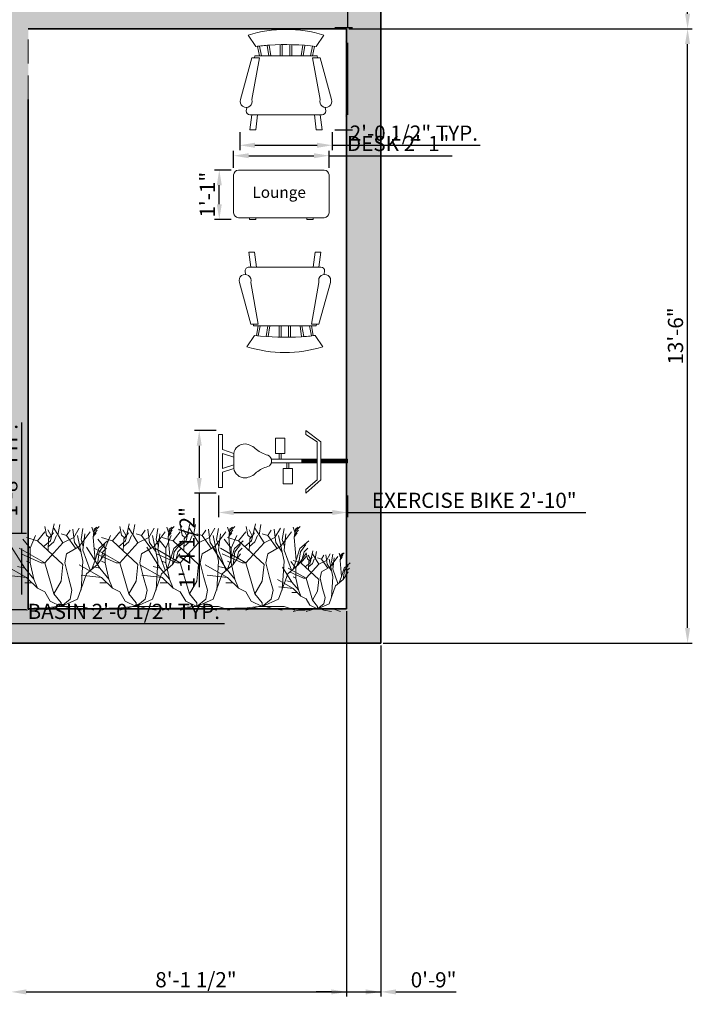
# Model space of a CAD drawing. Units: inches. Extents: x 1872 to 2380, y 714 to 1327.
# Tile 3 of 9: x 2200 to 2378, y 714 to 974. Entities that reach past the tile are written whole.
import ezdxf

# ---------------------------------------------------------------- set-up
doc = ezdxf.new("R2010")
doc.units = ezdxf.units.IN
doc.linetypes.add('HIDDEN', pattern=[9.525, 6.35, -3.175])
for name, color, linetype, lineweight in [('A-ANNO-DIMS', 2, 'Continuous', 18), ('A-AREA-IDEN', 7, 'Continuous', 18), ('A-EQPM', 8, 'Continuous', 18), ('A-FURN', 8, 'Continuous', 18), ('A-WALL', 7, 'Continuous', 35), ('A-WALL-HIDN', 7, 'HIDDEN', 18), ('L-PLNT', 3, 'Continuous', 13)]:
    doc.layers.add(name, color=color, linetype=linetype, lineweight=lineweight)
doc.layers.add('A-WALL-PATT', color=242, linetype='Continuous', lineweight=13, true_color=0xd52e31)
doc.styles.get("Standard").update_dxf_attribs({"font": 'arial.ttf'})
doc.dimstyles.new('ISO-25', dxfattribs={"dimtxt": 4, "dimasz": 4, "dimexe": 1.25, "dimexo": 0.625, "dimtad": 1, "dimdec": 0, "dimlunit": 3, "dimtxsty": 'Standard', "dimcen": 2.5, "dimadec": 0, "dimazin": 0, "dimtfac": 1, "dimtdec": 0, "dimtmove": 0, "dimatfit": 3, "dimfxl": 1, "dimarcsym": 0})

# ---------------------------------------------------------------- blocks, each defined once
blk = doc.blocks.new('*U18')
for p, q in [((-316.7634, 502.285), (-327.6092, 559.9176)), ((-286.512, 498.3226), (-307.4416, 538.0736)), ((-290.3982, 464.5406), (-265.6078, 577.8246)), ((-207.264, 451.104), (-268.224, 548.64)), ((-240.792, 502.285), (-228.3968, 573.8368)), ((-182.88, 499.872), (-158.496, 536.448)), ((-129.1844, 450.6214), (-140.0302, 542.036)), ((-134.112, 487.68), (-97.536, 548.64)), ((-85.7758, 472.4908), (-73.3552, 548.005)), ((-12.9032, 555.9552), (-2.0574, 522.1732)), ((-5.1562, 486.3846), (2.5908, 542.036)), ((-0.508, 508.254), (22.7584, 536.067)), ((1.0414, 526.1356), (35.1536, 559.9176)), ((2.5908, 542.036), (21.209, 555.9552)), ((-426.72, 414.528), (-475.488, 475.488)), ((-377.952, 463.296), (-451.104, 487.68)), ((-426.72, 414.528), (-390.144, 499.872)), ((-377.952, 463.296), (-329.184, 524.256)), ((-207.264, 304.8), (-377.952, 463.296)), ((-338.455, 424.7896), (-290.3982, 464.5406)), ((-296.5958, 484.4034), (-316.7634, 502.285)), ((-305.8922, 396.9512), (-302.7934, 478.4344)), ((-302.7934, 478.4344), (-270.256, 518.1854)), ((-268.7066, 458.5716), (-250.0884, 500.3038)), ((-182.88, 499.872), (-219.456, 512.064)), ((-207.264, 451.104), (-134.112, 487.68)), ((-121.92, 414.528), (-182.88, 499.872)), ((-73.152, 329.184), (-109.728, 499.872)), ((-97.536, 426.72), (-24.384, 524.256)), ((-70.2564, 426.7708), (-85.7758, 472.4908)), ((-73.152, 402.336), (-60.96, 512.064)), ((8.7884, 335.3562), (-5.1562, 486.3846)), ((-3.6068, 492.3536), (14.986, 518.1854)), ((33.6042, 412.8516), (92.5068, 464.5406)), ((-463.296, 280.416), (-552.577, 423.037)), ((-329.184, 316.992), (-499.872, 414.528)), ((-426.72, 316.992), (-426.72, 414.528)), ((-329.184, 316.992), (-207.264, 451.104)), ((-304.3428, 426.7708), (-268.7066, 458.5716)), ((-182.88, 377.952), (-97.536, 426.72)), ((-85.7758, 389.001), (-129.1844, 452.6026)), ((-24.384, 268.224), (-73.152, 402.336)), ((8.7884, 335.3562), (33.6042, 412.8516)), ((36.576, 390.144), (73.152, 438.912)), ((60.96, 390.144), (85.344, 414.528)), ((-353.568, 316.992), (-487.68, 377.952)), ((-195.072, 316.992), (-182.88, 377.952)), ((-12.192, 274.32), (8.7884, 335.3562)), ((24.384, 304.8), (36.576, 390.144)), ((24.384, 304.8), (73.152, 377.952)), ((48.768, 341.376), (60.96, 390.144)), ((-451.104, 219.456), (-601.0402, 303.8094)), ((-463.296, 280.416), (-512.064, 292.608)), ((-402.336, 207.264), (-463.296, 280.416)), ((-426.72, 316.992), (-451.104, 329.184)), ((-402.336, 207.264), (-426.72, 316.992)), ((-329.184, 316.992), (-353.568, 316.992)), ((-268.224, 109.728), (-329.184, 316.992)), ((-219.456, 195.072), (-207.264, 304.8)), ((-170.688, 219.456), (-195.072, 316.992)), ((-85.344, 134.112), (-73.152, 329.184)), ((-48.768, 243.84), (24.384, 304.8)), ((-451.104, 219.456), (-587.4512, 234.2388)), ((-377.952, 146.304), (-451.104, 219.456)), ((-377.952, 146.304), (-402.336, 207.264)), ((-146.304, 134.112), (-170.688, 219.456)), ((-109.728, 73.152), (-48.768, 243.84)), ((-414.528, 182.88), (-463.296, 182.88)), ((-329.184, 121.92), (-377.952, 146.304)), ((-268.224, 109.728), (-219.456, 195.072)), ((-158.496, 73.152), (-146.304, 134.112)), ((-292.608, 60.96), (-329.184, 121.92)), ((-219.456, 48.768), (-268.224, 109.728)), ((-219.456, 24.384), (-109.728, 73.152)), ((-219.456, 24.384), (-158.496, 73.152)), ((-402.336, 12.192), (-451.104, 0)), ((-341.376, 12.192), (-402.336, 12.192)), ((-243.84, 24.384), (-341.376, 12.192)), ((-243.84, 24.384), (-329.184, 0)), ((-219.456, 24.384), (-292.608, 60.96)), ((-243.84, 24.384), (-195.072, 24.384)), ((-219.456, 24.384), (-219.456, 48.768)), ((-219.456, 24.384), (-73.152, 24.384)), ((-195.072, 24.384), (-158.496, 12.192)), ((-158.496, 12.192), (-85.344, 0)), ((-73.152, 24.384), (0, 0))]:
    blk.add_line(p, q)
blk = doc.blocks.new('Desk - 30 x 60 in.')
for p, q in [((-26.999995, 0), (26.999995, 0)), ((-29.999995, -27), (-29.999995, -3)), ((29.999995, -3), (29.999995, -27)), ((26.999995, -30), (-26.999995, -30)), ((-20.000005, -30), (-20.000005, -31)), ((-16.000005, -31), (-16.000005, -30)), ((15.999995, -31), (15.999995, -30)), ((19.999995, -30), (19.999995, -31)), ((-20.000005, -31), (-16.000005, -31)), ((19.999995, -31), (15.999995, -31))]:
    blk.add_line(p, q)
for centre, start, end in [((-26.499995, -3.5), 98.1301, 171.8699), ((26.499995, -3.5), 8.130102, 81.8699), ((-26.499995, -26.5), 188.1301, 261.8699), ((26.499995, -26.5), 278.1301, 351.8699)]:
    blk.add_arc(centre, 3.535534, start, end)
blk = doc.blocks.new('Exercise Bike')
for p, q in [((-0.75, 10), (-0.75, 17)), ((-0.75, 17), (0.25, 17)), ((-0.5, 17), (-0.5, 9.9929)), ((-0.25, 10), (-0.25, 17)), ((0, 17), (0, 9.9929)), ((0.25, 17), (0.25, 10)), ((-5.25, 10), (-8.25, 6)), ((-7.25, 6), (-5.25, 9)), ((-0.75, 10), (-5.25, 10)), ((-5.25, 9), (4.75, 9)), ((4.75, 10), (-0.75, 10)), ((-0.75, 5), (-0.75, 9)), ((-0.5, 8.9396), (-0.5, 5)), ((-0.25, 5), (-0.25, 9)), ((0, 8.9396), (0, 5)), ((0.25, 9), (0.25, 5)), ((8.25, 6), (4.75, 10)), ((4.75, 9), (7.25, 6)), ((-8.25, 6), (-7.25, 6)), ((7.25, 6), (8.25, 6)), ((-0.75, -3.0635), (-0.75, 5)), ((-0.75, 5), (0.25, 5)), ((0.25, 5), (0.25, -3.0635)), ((-6.25, -2), (-6.25, 0.5)), ((-2.25, 0.5), (-6.25, 0.5)), ((-2.25, -0.5), (-2.25, 0.5)), ((0.25, 1.5), (1.75, 1.5)), ((0.25, 1), (1.75, 1)), ((1.75, 2.5), (5.75, 2.5)), ((1.75, 1.5), (1.75, 2.5)), ((1.75, 1.5), (1.75, 0)), ((1.75, 0), (5.75, 0)), ((5.75, 2.5), (5.75, 0)), ((-2.25, -2), (-6.25, -2)), ((-2.25, -0.5), (-0.75, -0.5)), ((-2.25, -1), (-2.25, -0.5)), ((-2.25, -1), (-2.25, -2)), ((-0.75, -1), (-2.25, -1)), ((-2.25, -13), (-3.25, -16)), ((-2.25, -16), (-1.25, -13)), ((-2.25, -13), (1.75, -13)), ((0.75, -13), (1.75, -16)), ((1.75, -13), (2.75, -16)), ((-7.25, -16), (-7.25, -17)), ((-4.75, -16), (-7.25, -16)), ((-7.25, -17), (6.75, -17)), ((-3.25, -16), (-4.75, -16)), ((1.75, -16), (-2.25, -16)), ((6.75, -16), (2.75, -16)), ((6.75, -17), (6.75, -16))]:
    blk.add_line(p, q)
for centre, radius, start, end in [((-9.6692, -1.9154), 8.1889, 321.6175, 345.2525), ((-0.25, -4.625), 1.625, 22.61987, 157.3801), ((9.1691, -1.9154), 8.1889, 194.7476, 218.3825), ((0.1685, -10.5843), 4.9531, 133.6443, 173.2256), ((-0.6686, -10.5843), 4.9531, 6.774486, 46.35562), ((-1.7006, -10.0005), 3.0494, 179.9906, 259.6205), ((1.2006, -10.0005), 3.0494, 280.3795, 0.009389)]:
    blk.add_arc(centre, radius, start, end)
blk = doc.blocks.new('Chair - Rocking')
for p, q in [((-8, -4.5), (-10, -1.5)), ((8, -4.5), (10, -1.5)), ((-7.5, -4.5), (-7, -7)), ((-6.5, -7), (-7.02225, -4.43)), ((-4.5, -7), (-4.96674, -4.19951)), ((-4, -7), (-4.40532, -4.16272)), ((-1.5, -4.05012), (-1.5, -7)), ((-1, -7), (-1, -4.05012)), ((1, -7), (1, -4.04655)), ((1.5, -4.05012), (1.5, -7)), ((4, -7), (4.40187, -4.18694)), ((4.5, -7), (4.96761, -4.19437)), ((6.5, -7), (7, -4.4057)), ((7.5, -4.5), (7, -7)), ((-9, -7.5), (-12, -18.49999)), ((-7, -7.5), (-9, -7.5)), ((-9, -18.49999), (-7, -7.5)), ((-8.23428, -6.99939), (-8.3093, -7.47958)), ((-8.23041, -7), (8.23915, -7)), ((7, -7.5), (9, -7.5)), ((9, -18.49999), (7, -7.5)), ((8.31071, -7.48854), (8.23449, -7.00073)), ((9, -7.5), (12, -18.49999)), ((-10.36644, -20.64523), (-10.5, -21.49999)), ((10.5, -21.49999), (10.3575, -20.58798)), ((-9, -22.49999), (-9.5, -26.49999)), ((0, -22.49999), (-9.5, -22.49999)), ((-8, -26.49999), (-7.5, -22.49999)), ((0, -22.49999), (9.5, -22.49999)), ((8, -26.49999), (7.5, -22.49999)), ((9, -22.49999), (9.5, -26.49999)), ((-9.5, -26.49999), (-8, -26.49999)), ((9.5, -26.49999), (8, -26.49999))]:
    blk.add_line(p, q)
for centre, radius, start, end in [((0, -34.08333), 34.08333, 72.93847, 107.0615), ((0, -68.25004), 64.25, 93.92211, 97.15267), ((0, -68.25004), 64.25, 82.84733, 93.92211), ((-10.5, -18.99999), 1.58114, 161.5651, 18.43495), ((10.5, -18.99999), 1.58114, 161.5651, 18.43495), ((-9.5, -21.49999), 1, 180, 270), ((9.5, -21.49999), 1, 270, 0)]:
    blk.add_arc(centre, radius, start, end)
blk = doc.blocks.new('*D30')
at = {"layer": 'A-ANNO-DIMS', "color": 0, "lineweight": -2, "transparency": 16777216}
for p, q in [((2172.51, 817.84), (2172.51, 813.54)), ((2197.06, 817.84), (2197.06, 813.54)), ((2176.51, 814.79), (2193.06, 814.79)), ((2197.06, 814.79), (2254.16, 814.79))]:
    blk.add_line(p, q, dxfattribs=at)
at = {"layer": 'A-ANNO-DIMS', "color": 0, "transparency": 16777216}
for points in [[(2176.51, 815.45), (2176.51, 814.12), (2172.51, 814.79)], [(2193.06, 815.45), (2193.06, 814.12), (2197.06, 814.79)]]:
    blk.add_solid(points, dxfattribs=at)
at = {"layer": 'Defpoints', "color": 0, "transparency": 16777216}
for p in [(2172.51, 818.47), (2197.06, 818.47), (2197.06, 814.79)]:
    blk.add_point(p, dxfattribs=at)
at = {"layer": 'A-ANNO-DIMS', "color": 0, "transparency": 16777216, "insert": (2227.61, 817.48), "char_height": 4, "attachment_point": 5}
blk.add_mtext('BASIN 2\'-0 1/2" TYP.', dxfattribs=at)
blk = doc.blocks.new('*D31')
at = {"layer": 'A-ANNO-DIMS', "color": 0, "lineweight": -2, "transparency": 16777216}
for p, q in [((2200.74, 838.61), (2200.74, 867.86)), ((2197.68, 838.61), (2201.99, 838.61)), ((2200.74, 822.47), (2200.74, 834.61)), ((2197.68, 818.47), (2201.99, 818.47))]:
    blk.add_line(p, q, dxfattribs=at)
at = {"layer": 'A-ANNO-DIMS', "color": 0, "transparency": 16777216}
for points in [[(2200.07, 834.61), (2201.41, 834.61), (2200.74, 838.61)], [(2200.07, 822.47), (2201.41, 822.47), (2200.74, 818.47)]]:
    blk.add_solid(points, dxfattribs=at)
at = {"layer": 'Defpoints', "color": 0, "transparency": 16777216}
for p in [(2197.06, 838.61), (2200.74, 838.61), (2197.06, 818.47)]:
    blk.add_point(p, dxfattribs=at)
at = {"layer": 'A-ANNO-DIMS', "color": 0, "transparency": 16777216, "insert": (2198.07, 855.23), "char_height": 4, "attachment_point": 5, "rotation": 90}
blk.add_mtext('1\'-8" TYP.', dxfattribs=at)
blk = doc.blocks.new('*D38')
at = {"layer": 'A-ANNO-DIMS', "color": 0, "lineweight": -2, "transparency": 16777216}
for p, q in [((2286.68, 972), (2286.68, 1026.88)), ((2283.25, 972), (2287.93, 972)), ((2286.68, 949), (2286.68, 968)), ((2283.25, 945), (2287.93, 945))]:
    blk.add_line(p, q, dxfattribs=at)
at = {"layer": 'A-ANNO-DIMS', "color": 0, "transparency": 16777216}
for points in [[(2286.01, 968), (2287.34, 968), (2286.68, 972)], [(2286.01, 949), (2287.34, 949), (2286.68, 945)]]:
    blk.add_solid(points, dxfattribs=at)
at = {"layer": 'Defpoints', "color": 0, "transparency": 16777216}
for p in [(2282.63, 972), (2286.68, 972), (2282.63, 945)]:
    blk.add_point(p, dxfattribs=at)
at = {"layer": 'A-ANNO-DIMS', "color": 0, "transparency": 16777216, "insert": (2283.98, 1001.44), "char_height": 4, "attachment_point": 5, "rotation": 90}
blk.add_mtext('ROCKER 2\'-3" TYP.', dxfattribs=at)
blk = doc.blocks.new('*D39')
at = {"layer": 'A-ANNO-DIMS', "color": 0, "lineweight": -2, "transparency": 16777216}
for p, q in [((2258.19, 944.37), (2258.19, 939.7)), ((2282.63, 944.37), (2282.63, 939.7)), ((2262.19, 940.95), (2278.63, 940.95)), ((2282.63, 940.95), (2321.65, 940.95))]:
    blk.add_line(p, q, dxfattribs=at)
at = {"layer": 'A-ANNO-DIMS', "color": 0, "transparency": 16777216}
for points in [[(2262.19, 941.62), (2262.19, 940.28), (2258.19, 940.95)], [(2278.63, 941.62), (2278.63, 940.28), (2282.63, 940.95)]]:
    blk.add_solid(points, dxfattribs=at)
at = {"layer": 'Defpoints', "color": 0, "transparency": 16777216}
for p in [(2258.19, 945), (2282.63, 945), (2282.63, 940.95)]:
    blk.add_point(p, dxfattribs=at)
at = {"layer": 'A-ANNO-DIMS', "color": 0, "transparency": 16777216, "insert": (2304.14, 943.64), "char_height": 4, "attachment_point": 5}
blk.add_mtext('2\'-0 1/2" TYP.', dxfattribs=at)
blk = doc.blocks.new('*D48')
at = {"layer": 'A-ANNO-DIMS', "color": 0, "lineweight": -2, "transparency": 16777216}
for p, q in [((2256.59, 935.04), (2256.59, 939.45)), ((2260.59, 938.2), (2277.77, 938.2)), ((2281.77, 935.04), (2281.77, 939.45)), ((2281.77, 938.2), (2314.22, 938.2))]:
    blk.add_line(p, q, dxfattribs=at)
at = {"layer": 'A-ANNO-DIMS', "color": 0, "transparency": 16777216}
for points in [[(2260.59, 938.86), (2260.59, 937.53), (2256.59, 938.2)], [(2277.77, 938.86), (2277.77, 937.53), (2281.77, 938.2)]]:
    blk.add_solid(points, dxfattribs=at)
at = {"layer": 'Defpoints', "color": 0, "transparency": 16777216}
for p in [(2281.77, 938.2), (2256.59, 934.42), (2281.77, 934.42)]:
    blk.add_point(p, dxfattribs=at)
at = {"layer": 'A-ANNO-DIMS', "color": 0, "transparency": 16777216, "insert": (2299.99, 940.89), "char_height": 4, "attachment_point": 5}
blk.add_mtext('DESK 2\'-1"', dxfattribs=at)
blk = doc.blocks.new('*D49')
at = {"layer": 'A-ANNO-DIMS', "color": 0, "lineweight": -2, "transparency": 16777216}
for p, q in [((2255.97, 934.42), (2251.56, 934.42)), ((2252.81, 925.41), (2252.81, 930.42)), ((2255.97, 921.41), (2251.56, 921.41))]:
    blk.add_line(p, q, dxfattribs=at)
at = {"layer": 'A-ANNO-DIMS', "color": 0, "transparency": 16777216}
for points in [[(2252.15, 930.42), (2253.48, 930.42), (2252.81, 934.42)], [(2252.15, 925.41), (2253.48, 925.41), (2252.81, 921.41)]]:
    blk.add_solid(points, dxfattribs=at)
at = {"layer": 'Defpoints', "color": 0, "transparency": 16777216}
for p in [(2252.81, 934.42), (2256.59, 934.42), (2256.59, 921.41)]:
    blk.add_point(p, dxfattribs=at)
at = {"layer": 'A-ANNO-DIMS', "color": 0, "transparency": 16777216, "insert": (2250.18, 927.91), "char_height": 4, "attachment_point": 5, "rotation": 90}
blk.add_mtext('1\'-1"', dxfattribs=at)
blk = doc.blocks.new('*D50')
at = {"layer": 'A-ANNO-DIMS', "color": 0, "lineweight": -2, "transparency": 16777216}
for p, q in [((2252.62, 848.56), (2252.62, 842.84)), ((2286.62, 848.56), (2286.62, 842.84)), ((2256.62, 844.09), (2282.62, 844.09)), ((2286.62, 844.09), (2349.5, 844.09))]:
    blk.add_line(p, q, dxfattribs=at)
at = {"layer": 'A-ANNO-DIMS', "color": 0, "transparency": 16777216}
for points in [[(2256.62, 844.75), (2256.62, 843.42), (2252.62, 844.09)], [(2282.62, 844.75), (2282.62, 843.42), (2286.62, 844.09)]]:
    blk.add_solid(points, dxfattribs=at)
at = {"layer": 'Defpoints', "color": 0, "transparency": 16777216}
for p in [(2252.62, 849.19), (2286.62, 849.19), (2286.62, 844.09)]:
    blk.add_point(p, dxfattribs=at)
at = {"layer": 'A-ANNO-DIMS', "color": 0, "transparency": 16777216, "insert": (2320.06, 846.78), "char_height": 4, "attachment_point": 5}
blk.add_mtext('EXERCISE BIKE 2\'-10"', dxfattribs=at)
blk = doc.blocks.new('*D51')
at = {"layer": 'A-ANNO-DIMS', "color": 0, "lineweight": -2, "transparency": 16777216}
for p, q in [((2252, 865.69), (2246.27, 865.69)), ((2247.52, 861.69), (2247.52, 853.19)), ((2252, 849.19), (2246.27, 849.19)), ((2247.52, 849.19), (2247.52, 824.36))]:
    blk.add_line(p, q, dxfattribs=at)
at = {"layer": 'A-ANNO-DIMS', "color": 0, "transparency": 16777216}
for points in [[(2246.86, 861.69), (2248.19, 861.69), (2247.52, 865.69)], [(2246.86, 853.19), (2248.19, 853.19), (2247.52, 849.19)]]:
    blk.add_solid(points, dxfattribs=at)
at = {"layer": 'Defpoints', "color": 0, "transparency": 16777216}
for p in [(2252.62, 865.69), (2247.52, 849.19), (2252.62, 849.19)]:
    blk.add_point(p, dxfattribs=at)
at = {"layer": 'A-ANNO-DIMS', "color": 0, "transparency": 16777216, "insert": (2244.83, 834.77), "char_height": 4, "attachment_point": 5, "rotation": 90}
blk.add_mtext('1\'-4 1/2"', dxfattribs=at)
blk = doc.blocks.new('*D61')
at = {"layer": 'A-ANNO-DIMS', "color": 0, "lineweight": -2, "transparency": 16777216}
for p, q in [((2197.9, 818.02), (2197.9, 716.39)), ((2295.4, 809.02), (2295.4, 716.39)), ((2201.9, 717.64), (2291.4, 717.64))]:
    blk.add_line(p, q, dxfattribs=at)
at = {"layer": 'A-ANNO-DIMS', "color": 0, "transparency": 16777216}
for points in [[(2201.9, 718.3), (2201.9, 716.97), (2197.9, 717.64)], [(2291.4, 718.3), (2291.4, 716.97), (2295.4, 717.64)]]:
    blk.add_solid(points, dxfattribs=at)
at = {"layer": 'Defpoints', "color": 0, "transparency": 16777216}
for p in [(2197.9, 818.64), (2295.4, 809.64), (2295.4, 717.64)]:
    blk.add_point(p, dxfattribs=at)
at = {"layer": 'A-ANNO-DIMS', "color": 0, "transparency": 16777216, "insert": (2246.65, 720.33), "char_height": 4, "attachment_point": 5}
blk.add_mtext('8\'-1 1/2"', dxfattribs=at)
blk = doc.blocks.new('*D62')
at = {"layer": 'A-ANNO-DIMS', "color": 0, "lineweight": -2, "transparency": 16777216}
for p, q in [((2287.02, 971.64), (2377.6, 971.64)), ((2376.35, 813.64), (2376.35, 967.64)), ((2296.02, 809.64), (2377.6, 809.64))]:
    blk.add_line(p, q, dxfattribs=at)
at = {"layer": 'A-ANNO-DIMS', "color": 0, "transparency": 16777216}
for points in [[(2375.68, 967.64), (2377.01, 967.64), (2376.35, 971.64)], [(2375.68, 813.64), (2377.01, 813.64), (2376.35, 809.64)]]:
    blk.add_solid(points, dxfattribs=at)
at = {"layer": 'Defpoints', "color": 0, "transparency": 16777216}
for p in [(2286.4, 971.64), (2376.35, 971.64), (2295.4, 809.64)]:
    blk.add_point(p, dxfattribs=at)
at = {"layer": 'A-ANNO-DIMS', "color": 0, "transparency": 16777216, "insert": (2373.68, 890.64), "char_height": 4, "attachment_point": 5, "rotation": 90}
blk.add_mtext('13\'-6"', dxfattribs=at)
blk = doc.blocks.new('*D63')
at = {"layer": 'A-ANNO-DIMS', "color": 0, "lineweight": -2, "transparency": 16777216}
for p, q in [((2287.02, 1055.64), (2377.6, 1055.64)), ((2376.35, 975.64), (2376.35, 1051.64)), ((2287.02, 971.64), (2377.6, 971.64))]:
    blk.add_line(p, q, dxfattribs=at)
at = {"layer": 'A-ANNO-DIMS', "color": 0, "transparency": 16777216}
for points in [[(2375.68, 1051.64), (2377.01, 1051.64), (2376.35, 1055.64)], [(2375.68, 975.64), (2377.01, 975.64), (2376.35, 971.64)]]:
    blk.add_solid(points, dxfattribs=at)
at = {"layer": 'Defpoints', "color": 0, "transparency": 16777216}
for p in [(2286.4, 1055.64), (2376.35, 1055.64), (2286.4, 971.64)]:
    blk.add_point(p, dxfattribs=at)
at = {"layer": 'A-ANNO-DIMS', "color": 0, "transparency": 16777216, "insert": (2373.68, 1013.64), "char_height": 4, "attachment_point": 5, "rotation": 90}
blk.add_mtext('7\'-0"', dxfattribs=at)
blk = doc.blocks.new('*D79')
at = {"layer": 'A-ANNO-DIMS', "color": 0, "lineweight": -2, "transparency": 16777216}
for p, q in [((2286.4, 818.02), (2286.4, 716.39)), ((2295.4, 809.02), (2295.4, 716.39)), ((2282.4, 717.64), (2278.4, 717.64)), ((2286.4, 717.64), (2295.4, 717.64)), ((2299.4, 717.64), (2315.28, 717.64))]:
    blk.add_line(p, q, dxfattribs=at)
at = {"layer": 'A-ANNO-DIMS', "color": 0, "transparency": 16777216}
for points in [[(2282.4, 718.3), (2282.4, 716.97), (2286.4, 717.64)], [(2299.4, 718.3), (2299.4, 716.97), (2295.4, 717.64)]]:
    blk.add_solid(points, dxfattribs=at)
at = {"layer": 'Defpoints', "color": 0, "transparency": 16777216}
for p in [(2286.4, 818.64), (2295.4, 809.64), (2295.4, 717.64)]:
    blk.add_point(p, dxfattribs=at)
at = {"layer": 'A-ANNO-DIMS', "color": 0, "transparency": 16777216, "insert": (2309.34, 720.31), "char_height": 4, "attachment_point": 5}
blk.add_mtext('0\'-9"', dxfattribs=at)

msp = doc.modelspace()

# ---------------------------------------------------------------- hatches: boundary and pattern name
at = {"layer": 'A-WALL-PATT', "transparency": 33554687}
h = msp.add_hatch(color=256, dxfattribs=at)
h.dxf.hatch_style = 1
h.paths.add_polyline_path([(2295.4, 1289.64), (1935.4, 1289.64), (1935.4, 809.64), (1949.4, 809.64), (1949.4, 818.64), (1944.4, 818.64), (1944.4, 1108.27), (2100.4, 1108.27), (2100.4, 1112.77), (1944.4, 1112.77), (1944.4, 1280.64), (2095.9, 1280.64), (2095.9, 1141.77), (2100.4, 1141.77), (2100.4, 1280.64), (2169.91, 1280.64), (2169.91, 1244.64), (2169.91, 1160.49, -0.053008), (2170.04, 1158.75, -0.03687), (2169.91, 1157.54), (2169.91, 1148.64), (2167.91, 1148.64), (2138.4, 1148.64), (2138.4, 1144.14), (2167.91, 1144.14), (2174.41, 1144.14), (2174.41, 1280.64), (2197.9, 1280.64), (2197.9, 1184.64), (2202.4, 1184.64), (2202.4, 1280.64), (2286.4, 1280.64), (2286.4, 1148.64), (2197.9, 1148.64), (2197.9, 1108.14), (2202.4, 1108.14), (2202.4, 1144.14), (2286.4, 1144.14), (2286.4, 1060.14), (2202.4, 1060.14), (2202.4, 1108.14), (2197.9, 1108.14), (2197.9, 1060.14), (2197.9, 1053.64), (2202.4, 1053.64), (2202.4, 1055.64), (2286.4, 1055.64), (2286.4, 976.14), (2202.4, 976.14), (2202.4, 1015.64), (2197.9, 1015.64), (2197.9, 971.64), (2197.9, 952.99), (2197.9, 818.64), (2101.9, 818.64), (2101.9, 948.71), (2130.4, 948.71), (2130.4, 952.99), (2073.4, 952.99), (2073.4, 948.71), (2097.4, 948.71), (2097.4, 818.64), (2005.9, 818.64), (2005.9, 948.71), (2029.9, 948.71), (2029.9, 952.99), (2001.4, 952.99), (2001.4, 818.64), (1996.4, 818.64), (1985.23, 818.64), (1985.23, 809.64), (1996.4, 809.64), (2295.4, 809.64)])
h.paths.add_polyline_path([(2202.4, 971.64), (2286.4, 971.64), (2286.4, 858.19), (2286.62, 858.19), (2286.62, 857.19), (2286.4, 857.19), (2286.4, 828.68), (2286.48, 828.76), (2286.4, 828.43), (2286.4, 818.64), (2256.29, 818.64), (2255.29, 818.39), (2254.54, 818.64), (2238.99, 818.64), (2238.75, 818.58), (2238.56, 818.64), (2202.4, 818.64), (2202.4, 952.99)], flags=16)
h.paths.add_polyline_path([(2260.41, 970, -0.15), (2280.41, 970), (2278.41, 967, 0.001913), (2277.92, 967.06), (2277.41, 964.5), (2278.64, 964.5), (2278.72, 964), (2279.41, 964), (2282.41, 953, -0.541163), (2280.76, 950.93), (2280.91, 950, -0.414214), (2279.91, 949), (2279.41, 949), (2279.91, 945), (2278.41, 945), (2277.91, 949), (2270.41, 949), (2262.91, 949), (2262.41, 945), (2260.91, 945), (2261.41, 949), (2260.91, 949, -0.414214), (2259.91, 950), (2260.05, 950.93, -0.505809), (2258.36, 952.83), (2261.41, 964), (2262.1, 964), (2262.17, 964.5), (2263.41, 964.5), (2262.9, 967.06, 0.001913), (2262.41, 967)], flags=0)
h.paths.add_polyline_path([(2257.85, 934.42), (2280.51, 934.42, -0.333333), (2281.77, 933.16), (2281.77, 923.09, -0.333333), (2280.51, 921.83), (2277.57, 921.83), (2277.57, 921.41), (2275.89, 921.41), (2275.89, 921.83), (2262.46, 921.83), (2262.46, 921.41), (2260.79, 921.41), (2260.79, 921.83), (2257.85, 921.83, -0.333333), (2256.59, 923.09), (2256.59, 933.16, -0.333333)], flags=0)
h.paths.add_polyline_path([(2260.61, 912.79), (2262.11, 912.79), (2262.61, 908.79), (2270.11, 908.79), (2277.61, 908.79), (2278.11, 912.79), (2279.61, 912.79), (2279.11, 908.79), (2279.61, 908.79, -0.414214), (2280.61, 907.79), (2280.46, 906.86, -0.505809), (2282.15, 904.96), (2279.11, 893.79), (2278.42, 893.79), (2278.34, 893.29), (2277.11, 893.29), (2277.62, 890.73, 0.001913), (2278.11, 890.79), (2280.11, 887.79, -0.15), (2260.11, 887.79), (2262.11, 890.79, 0.001913), (2262.59, 890.73), (2263.11, 893.29), (2261.87, 893.29), (2261.79, 893.79), (2261.11, 893.79), (2258.11, 904.79, -0.541163), (2259.75, 906.86), (2259.61, 907.79, -0.414214), (2260.61, 908.79), (2261.11, 908.79)], flags=0)
h.paths.add_polyline_path([(2252.62, 864.69), (2253.62, 864.69), (2253.62, 862.19), (2253.62, 860.69), (2256.62, 859.69, -0.362186), (2259.62, 862.19, -0.174416), (2262.62, 860.69, 0.103487), (2265.62, 859.19, -0.219276), (2266.55, 858.19), (2268.62, 858.19), (2268.62, 859.69), (2267.62, 859.69), (2267.62, 863.69), (2270.12, 863.69), (2270.12, 859.69), (2269.12, 859.69), (2269.12, 858.19), (2274.62, 858.19), (2278.62, 858.19), (2278.62, 862.69), (2275.62, 864.69), (2275.62, 865.69), (2279.62, 862.69), (2279.62, 858.19), (2279.62, 852.69), (2275.62, 849.19), (2275.62, 850.19), (2278.62, 852.69), (2278.62, 857.19), (2274.62, 857.19), (2271.12, 857.19), (2271.12, 855.69), (2272.12, 855.69), (2272.12, 851.69), (2269.62, 851.69), (2269.62, 855.69), (2270.62, 855.69), (2270.62, 857.19), (2266.55, 857.19, -0.219162), (2265.62, 856.19, 0.103506), (2262.62, 854.69, -0.174459), (2259.62, 853.19, -0.362114), (2256.62, 855.69), (2253.62, 854.69), (2253.62, 850.69), (2252.62, 850.69)], flags=0)
h.paths.add_polyline_path([(2253.62, 859.69), (2256.62, 858.69), (2256.62, 856.69), (2253.62, 855.69)], flags=0)
h.paths.add_polyline_path([(2208.62, 838.17), (2208.28, 836.61), (2207.75, 836.18), (2207.67, 833.93), (2208.71, 832.96), (2211.55, 836.09), (2214.43, 837.53), (2214.45, 837.55), (2214.61, 836.16), (2215.48, 834.9), (2215.87, 835.13), (2217.12, 836.79), (2216.83, 834.17), (2218.8, 828.76), (2219.23, 829.13), (2220.06, 831.53), (2219.5, 837.61), (2219.53, 837.66), (2219.68, 838.72), (2219.62, 838.91), (2219.72, 839.01), (2219.51, 837.47), (2219.77, 834.68), (2220.87, 834.05), (2221.03, 834.58), (2222.05, 835.47), (2222.71, 834.65), (2223.67, 836.89), (2224.63, 836.57), (2226.23, 835.08), (2227.55, 836.18), (2227.59, 837.16), (2228.42, 838.17), (2228.08, 836.61), (2227.55, 836.18), (2227.47, 833.93), (2228.51, 832.96), (2231.35, 836.09), (2234.23, 837.53), (2234.25, 837.55), (2234.42, 836.16), (2235.28, 834.9), (2235.67, 835.13), (2236.93, 836.79), (2236.93, 836.84), (2238.69, 834.65), (2239.41, 836.34), (2239.3, 837.61), (2239.34, 837.66), (2239.48, 838.72), (2239.42, 838.91), (2239.52, 839.01), (2239.31, 837.47), (2239.36, 836.98), (2240.61, 836.57), (2242.2, 835.08), (2243.53, 836.18), (2243.57, 837.16), (2244.39, 838.17), (2244.05, 836.61), (2243.53, 836.18), (2243.44, 833.93), (2244.49, 832.96), (2247.33, 836.09), (2250.21, 837.53), (2250.22, 837.55), (2250.39, 836.16), (2251.25, 834.9), (2251.65, 835.13), (2252.9, 836.79), (2252.61, 834.17), (2254.09, 830.08), (2254.54, 829.37), (2254.85, 828.99), (2255.01, 829.13), (2255.83, 831.53), (2255.29, 837.44), (2255.28, 837.44), (2255.46, 838.72), (2255.4, 838.91), (2255.5, 839.01), (2255.28, 837.47), (2255.29, 837.44), (2257.9, 836.57), (2259.5, 835.08), (2260.82, 836.18), (2260.86, 837.16), (2261.69, 838.17), (2261.35, 836.61), (2260.82, 836.18), (2260.74, 833.93), (2261.78, 832.96), (2264.62, 836.09), (2267.5, 837.53), (2267.52, 837.55), (2267.68, 836.16), (2268.54, 834.9), (2268.94, 835.13), (2270.19, 836.79), (2269.9, 834.17), (2271.79, 828.96), (2271.98, 828.86), (2272.3, 829.13), (2273.13, 831.53), (2272.56, 837.61), (2272.6, 837.66), (2272.75, 838.72), (2272.69, 838.91), (2272.79, 839.01), (2272.58, 837.47), (2273.13, 831.53), (2273.02, 831.22), (2273.67, 831.01), (2273.92, 831.6), (2273.83, 830.95), (2274.1, 830.86), (2275.75, 833.35), (2276.03, 831.86), (2276.57, 831.38), (2277, 831.91), (2277.3, 833.27), (2279.06, 830.44), (2281.09, 831.46), (2281.1, 831.48), (2281.21, 830.5), (2281.82, 829.61), (2282.1, 829.77), (2282.98, 830.94), (2282.77, 829.1), (2284.15, 825.3), (2284.46, 825.55), (2285.04, 827.24), (2284.64, 831.51), (2284.67, 831.55), (2284.77, 832.3), (2284.73, 832.43), (2284.8, 832.5), (2284.65, 831.42), (2285.04, 827.24), (2284.46, 825.55), (2283.45, 824.71), (2281.76, 819.99), (2278.73, 818.64), (2276.7, 819.65), (2275.69, 821.34), (2274.34, 822.01), (2272.32, 824.04), (2269.58, 824.33), (2268.46, 821.21), (2264.14, 819.29), (2261.26, 820.73), (2259.82, 823.13), (2257.9, 824.09), (2255.02, 826.97), (2253.29, 827.15), (2251.17, 821.21), (2246.85, 819.29), (2243.97, 820.73), (2242.53, 823.13), (2240.61, 824.09), (2237.73, 826.97), (2237.27, 827.01), (2235.19, 821.21), (2230.87, 819.29), (2227.99, 820.73), (2226.55, 823.13), (2224.63, 824.09), (2221.75, 826.97), (2217.61, 827.41), (2215.39, 821.21), (2211.07, 819.29), (2208.19, 820.73), (2206.75, 823.13), (2204.83, 824.09), (2203.87, 826.49), (2202.91, 830.81), (2202.91, 834.65), (2203.87, 836.89), (2204.83, 836.57), (2206.43, 835.08), (2207.75, 836.18), (2207.79, 837.16)], flags=0)
h.paths.add_polyline_path([(2221.04, 832.88), (2221.82, 832.52), (2222.11, 833.69), (2222.71, 834.29), (2222.71, 832.11), (2225.59, 830.81), (2226.55, 830.81), (2228.95, 822.65), (2230.87, 820.25), (2230.87, 819.29), (2233.27, 821.21), (2233.75, 823.61), (2232.79, 826.97), (2231.99, 830.19), (2236.41, 827.71), (2236.63, 831.29), (2235.93, 834.58), (2242.53, 830.81), (2241.57, 830.81), (2240.97, 831.07), (2240.47, 830.33), (2239.06, 829.14), (2239.65, 826.49), (2237.25, 829.37), (2236.52, 829.55), (2236.41, 827.71), (2231.99, 830.19), (2232.79, 826.97), (2233.75, 823.61), (2233.27, 821.21), (2230.87, 819.29), (2230.87, 820.25), (2228.95, 822.65), (2226.55, 830.81), (2225.59, 830.81), (2222.71, 832.11), (2222.71, 830.81), (2223.67, 826.49), (2221.27, 829.37), (2220.67, 830.33), (2220.67, 830.33)], flags=0)
h.paths.add_polyline_path([(2255.98, 833), (2259.82, 830.81), (2258.86, 830.81), (2257.25, 831.54), (2256.45, 830.33), (2256.66, 831.81), (2256.02, 832.1), (2255.98, 831.99)], flags=0)
h.paths.add_polyline_path([(2275.69, 826.73), (2277.07, 828.25), (2275.46, 829.74), (2276.39, 830.51), (2276.33, 828.93), (2279.06, 826.4), (2278.73, 823.36), (2277.38, 821)], flags=0)
h.paths.add_polyline_path([(2260.6, 925.25), (2276.34, 925.25), (2276.34, 931.01), (2260.6, 931.01)], flags=8)
h.paths.add_polyline_path([(2202.72, 1070.05), (2202.72, 1092.72), (2197.34, 1092.72), (2197.34, 1070.05)], flags=25)

# ---------------------------------------------------------------- linework, layer by layer
at = {"layer": 'A-WALL'}
for p, q in [((2202.4, 971.64), (2286.4, 971.64)), ((2286.4, 818.64), (2202.4, 818.64))]:
    msp.add_line(p, q, dxfattribs=at)
at = {"layer": 'A-WALL', "transparency": 33554687}
for p, q in [((2286.4, 971.64), (2286.4, 818.64)), ((2202.4, 952.99), (2202.4, 818.64))]:
    msp.add_line(p, q, dxfattribs=at)
msp.add_lwpolyline([(1949.4, 809.64), (1935.4, 809.64), (1935.4, 1289.64), (2295.4, 1289.64), (2295.4, 809.64), (1996.4, 809.64)], dxfattribs=at)
at = {"layer": 'A-WALL-HIDN', "transparency": 33554687}
msp.add_line((2202.4, 952.99), (2202.4, 971.64), dxfattribs=at)

# ---------------------------------------------------------------- block references
at = {"layer": 'A-EQPM', "transparency": 33554687, "rotation": 270}
msp.add_blockref('Exercise Bike', (2269.62, 857.44), dxfattribs=at)
at = {"layer": 'A-FURN', "transparency": 33554687}
msp.add_blockref('Chair - Rocking', (2270.41, 971.5), dxfattribs=at)
at = {"layer": 'A-FURN', "transparency": 33554687, "xscale": 0.4196081032737203, "yscale": 0.4196081032737203, "zscale": 0.4196081032737203}
msp.add_blockref('Desk - 30 x 60 in.', (2269.18, 934.42), dxfattribs=at)
at = {"layer": 'A-FURN', "transparency": 33554687, "rotation": 180}
msp.add_blockref('Chair - Rocking', (2270.11, 886.29), dxfattribs=at)
at = {"layer": 'L-PLNT', "transparency": 33554687}
for p, xscale, yscale, zscale in [((2219.71, 818.33), 0.0393700787401575, 0.0393700787401575, 0.0393700787401575), ((2239.51, 818.33), 0.0393700787401575, 0.0393700787401575, 0.0393700787401575), ((2255.49, 818.33), 0.0393700787401575, 0.0393700787401575, 0.0393700787401575), ((2272.78, 818.33), 0.0393700787401575, 0.0393700787401575, 0.0393700787401575), ((2284.8, 817.97), 0.027658513280845, 0.027658513280845, 0.027658513280845)]:
    msp.add_blockref('*U18', p, dxfattribs=dict(at, xscale=xscale, yscale=yscale, zscale=zscale))

# ---------------------------------------------------------------- texts
at = {"layer": 'A-AREA-IDEN', "transparency": 33554687}
msp.add_text('Lounge', height=2.965, dxfattribs=at).set_placement((2261.56, 927.08))

# ---------------------------------------------------------------- dimensions: what is measured, and where the dimension line sits
at = {"layer": 'A-ANNO-DIMS', "transparency": 33554687}
for base, p1, p2, angle, picture, middle in [((2376.35, 1055.64), (2286.4, 971.64), (2286.4, 1055.64), 90, '*D63', (2373.68, 1013.64)), ((2376.35, 971.64), (2295.4, 809.64), (2286.4, 971.64), 90, '*D62', (2373.68, 890.64)), ((2252.81, 934.42), (2256.59, 921.41), (2256.59, 934.42), 90, '*D49', (2250.18, 927.91)), ((2247.52, 849.19), (2252.62, 865.69), (2252.62, 849.19), 270, '*D51', (2244.83, 834.77))]:
    dim = msp.add_linear_dim(base=base, p1=p1, p2=p2, angle=angle, dimstyle='ISO-25', override={"dimdec": 1, "dimlfac": 1, "dimrnd": 0, "dimzin": 1, "dimdsep": 46, "dimlunit": 4, "dimfrac": 2}, dxfattribs=at)
    dim.commit()
    dim.dimension.update_dxf_attribs({"geometry": picture, "text_midpoint": middle})
for base, p1, p2, text, picture, middle in [((2286.68, 972), (2282.63, 945), (2282.63, 972), 'ROCKER <> TYP.', '*D38', (2283.98, 1001.44)), ((2200.74, 838.61), (2197.06, 818.47), (2197.06, 838.61), '<> TYP.', '*D31', (2198.07, 855.23))]:
    dim = msp.add_linear_dim(base=base, p1=p1, p2=p2, angle=90, text=text, dimstyle='ISO-25', override={"dimdec": 1, "dimlfac": 1, "dimrnd": 0, "dimzin": 1, "dimdsep": 46, "dimlunit": 4, "dimfrac": 2}, dxfattribs=at)
    dim.commit()
    dim.dimension.update_dxf_attribs({"geometry": picture, "text_midpoint": middle})
for base, p1, p2, text, picture, middle in [((2282.63, 940.95), (2258.19, 945), (2282.63, 945), '<> TYP.', '*D39', (2304.14, 943.64)), ((2281.77, 938.2), (2256.59, 934.42), (2281.77, 934.42), 'DESK <>', '*D48', (2299.99, 940.89)), ((2286.62, 844.09), (2252.62, 849.19), (2286.62, 849.19), 'EXERCISE BIKE <>', '*D50', (2320.06, 846.78)), ((2197.0578, 814.7862), (2172.5069, 818.4689), (2197.0578, 818.4689), 'BASIN <> TYP.', '*D30', (2227.6064, 817.4794))]:
    dim = msp.add_linear_dim(base=base, p1=p1, p2=p2, text=text, dimstyle='ISO-25', override={"dimdec": 1, "dimlfac": 1, "dimrnd": 0, "dimzin": 1, "dimdsep": 46, "dimlunit": 4, "dimfrac": 2}, dxfattribs=at)
    dim.commit()
    dim.dimension.update_dxf_attribs({"geometry": picture, "text_midpoint": middle})
for p1, picture, middle in [((2197.9, 818.64), '*D61', (2246.65, 720.33)), ((2286.4, 818.64), '*D79', (2309.34, 720.31))]:
    dim = msp.add_linear_dim(base=(2295.4, 717.64), p1=p1, p2=(2295.4, 809.64), dimstyle='ISO-25', override={"dimdec": 1, "dimlfac": 1, "dimrnd": 0, "dimzin": 1, "dimdsep": 46, "dimlunit": 4, "dimfrac": 2}, dxfattribs=at)
    dim.commit()
    dim.dimension.update_dxf_attribs({"geometry": picture, "text_midpoint": middle})

doc.saveas('drawing.dxf')
